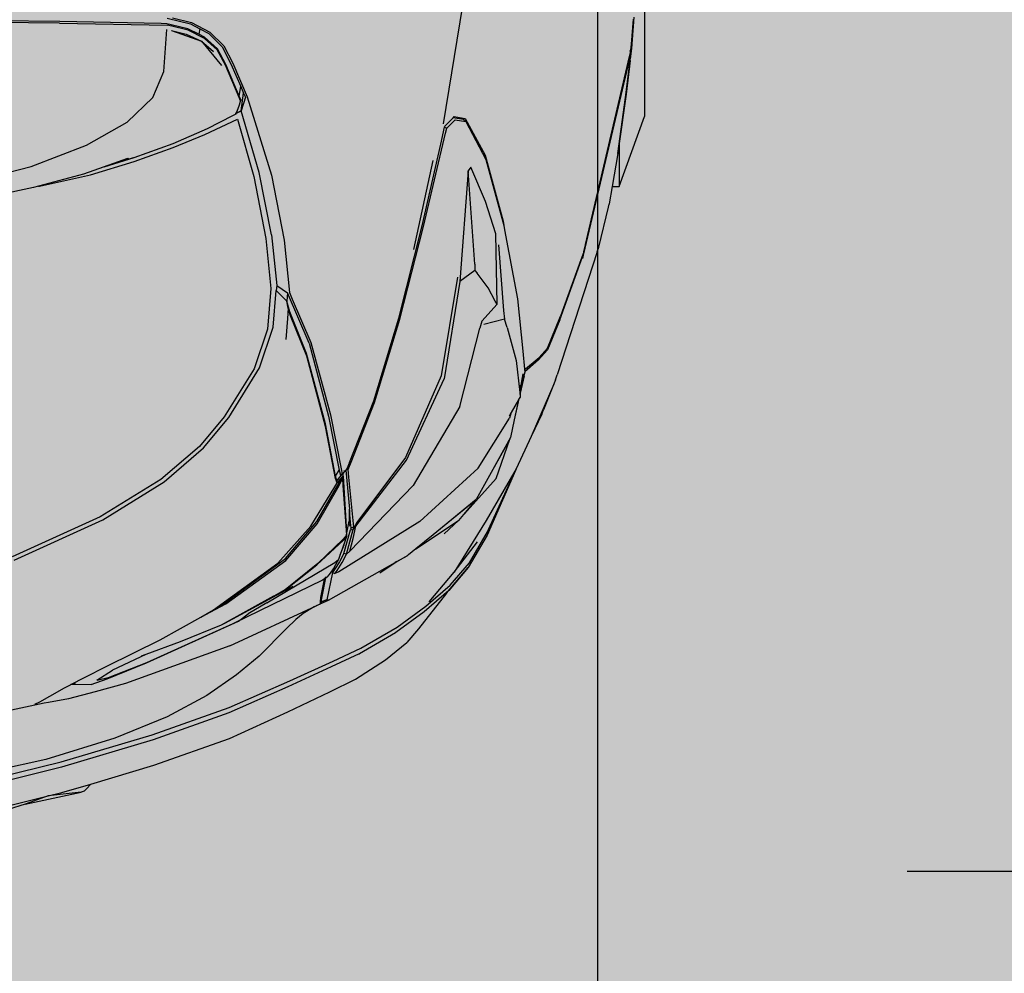
# Model space of a CAD drawing. Units: inches. Extents: x 1884 to 2398, y 474 to 1488.
# Tile 8 of 39: x 2247 to 2275, y 577 to 604. Entities that reach past the tile are written whole.
import ezdxf

# ---------------------------------------------------------------- set-up
doc = ezdxf.new("R2010")
doc.units = ezdxf.units.IN
doc.header["$MEASUREMENT"] = 0
doc.layers.get('0').update_dxf_attribs({"color": 250})
doc.layers.add('A-ANNO-DIMS', color=2, linetype='Continuous', lineweight=18)
doc.layers.add('C-VEHI', color=8, linetype='Continuous', lineweight=18)
doc.layers.add('Edges', color=250, linetype='Continuous')
doc.layers.add('L-PVMT-PATT', color=9, linetype='Continuous', lineweight=13, true_color=0xc7c8ca)
doc.styles.get("Standard").update_dxf_attribs({"font": 'arial.ttf'})
doc.dimstyles.get("Standard").update_dxf_attribs({"dimtxt": 7, "dimasz": 0.18, "dimexe": 0.18, "dimexo": 0.0625, "dimgap": 0.09, "dimtad": 0, "dimtih": 1, "dimtoh": 1, "dimzin": 0, "dimdsep": 46, "dimlunit": 3, "dimtxsty": 'Standard', "dimcen": 0.09, "dimadec": 0, "dimazin": 0, "dimtfac": 1, "dimtofl": 0, "dimtmove": 0, "dimatfit": 3, "dimfxl": 1, "dimtolj": 1, "dimtzin": 0, "dimarcsym": 0})

# ---------------------------------------------------------------- blocks, each defined once
blk = doc.blocks.new('Nissan Qashqai pl')
at = {"layer": 'Edges'}
for p, q in [((10.95774, 12.81008), (11.12826, 12.81008)), ((11.17826, 12.79208), (11.12826, 12.81008)), ((11.05762, 12.80257), (11.07977, 12.80077)), ((11.07681, 12.80079), (11.05899, 12.80228)), ((11.08106, 12.80045), (11.07681, 12.80079)), ((11.07977, 12.80077), (11.08723, 12.79991)), ((11.08273, 12.80006), (11.08106, 12.80045)), ((11.08273, 12.80006), (11.08133, 12.79984)), ((11.08365, 12.80022), (11.08273, 12.80006)), ((11.08562, 12.7994), (11.08273, 12.80006)), ((11.08723, 12.79991), (11.08365, 12.80022)), ((11.08365, 12.80022), (11.08821, 12.79916)), ((11.21955, 12.76812), (11.08562, 12.7994)), ((11.08834, 12.79978), (11.08723, 12.79991)), ((11.08821, 12.79916), (11.2222, 12.7676)), ((11.08834, 12.79978), (11.11234, 12.797)), ((11.11474, 12.79654), (11.08834, 12.79978)), ((11.11234, 12.797), (11.14751, 12.79208)), ((11.15472, 12.79099), (11.11474, 12.79654)), ((11.14751, 12.79208), (11.15248, 12.79138)), ((11.14751, 12.79208), (11.17826, 12.79208)), ((11.15248, 12.79138), (11.15472, 12.79099)), ((11.15472, 12.79099), (11.17826, 12.78701)), ((11.17826, 12.78701), (11.17826, 12.79208)), ((11.17826, 12.78701), (11.19065, 12.78493)), ((11.19065, 12.78493), (11.19089, 12.78487)), ((11.19297, 12.78452), (11.19089, 12.78487)), ((11.22148, 12.77754), (11.19297, 12.78452)), ((11.22475, 12.77644), (11.22148, 12.77754)), ((11.22475, 12.77644), (11.31244, 12.74788)), ((11.2247, 12.76695), (11.21633, 12.76893)), ((11.21998, 12.76802), (11.21955, 12.76812)), ((11.2247, 12.76695), (11.21998, 12.76802)), ((11.2222, 12.7676), (11.22715, 12.76645)), ((11.22532, 12.76679), (11.2247, 12.76695)), ((11.23038, 12.76493), (11.22532, 12.76679)), ((11.22532, 12.76679), (11.22706, 12.76639)), ((11.22715, 12.76645), (11.22962, 12.76579)), ((11.22715, 12.76645), (11.22772, 12.76624)), ((11.22772, 12.76624), (11.22962, 12.76579)), ((11.2732, 12.74964), (11.22772, 12.76624)), ((11.27044, 12.75036), (11.23038, 12.76493)), ((11.27015, 12.75067), (11.27044, 12.75036)), ((11.27037, 12.7506), (11.27066, 12.75028)), ((11.27066, 12.75028), (11.27044, 12.75036)), ((11.27187, 12.74984), (11.27066, 12.75028)), ((11.29339, 12.74103), (11.27187, 12.74984)), ((11.2732, 12.74964), (11.29459, 12.74089)), ((11.31612, 12.74669), (11.31244, 12.74788)), ((11.31612, 12.74669), (11.33757, 12.73813)), ((11.31923, 12.74536), (11.35656, 12.7294)), ((11.30003, 12.735), (11.29339, 12.74103)), ((11.29459, 12.74089), (11.30178, 12.73455)), ((11.30813, 12.72533), (11.30003, 12.735)), ((11.30178, 12.73455), (11.31027, 12.72493)), ((11.34052, 12.73691), (11.33757, 12.73813)), ((11.34052, 12.73691), (11.35656, 12.7294)), ((11.35656, 12.7294), (11.37962, 12.71869)), ((11.25827, 12.71956), (11.29558, 12.72339)), ((11.29558, 12.72339), (11.30849, 12.72466)), ((11.30218, 12.71856), (11.32517, 12.7213)), ((11.30863, 12.72468), (11.30813, 12.72533)), ((11.30813, 12.72533), (11.30866, 12.72468)), ((11.30849, 12.72466), (11.30863, 12.72468)), ((11.30863, 12.72468), (11.30866, 12.72468)), ((11.30866, 12.72468), (11.31033, 12.72486)), ((11.31027, 12.72493), (11.31033, 12.72486)), ((11.31033, 12.72486), (11.31061, 12.72489)), ((11.31061, 12.72489), (11.314, 12.72377)), ((11.31704, 12.72274), (11.31186, 12.72358)), ((11.31323, 12.7243), (11.32564, 12.72151)), ((11.314, 12.72377), (11.31704, 12.72274)), ((11.314, 12.72377), (11.32423, 12.72158)), ((11.32423, 12.72158), (11.31704, 12.72274)), ((11.31982, 12.72106), (11.32517, 12.7213)), ((11.32423, 12.72158), (11.32564, 12.72151)), ((11.32517, 12.7213), (11.32831, 12.72138)), ((11.32564, 12.72151), (11.32831, 12.72138)), ((11.32831, 12.72138), (11.32971, 12.7206)), ((11.32971, 12.7206), (11.34455, 12.71727)), ((11.32971, 12.7206), (11.33021, 12.72032)), ((11.33021, 12.72032), (11.34455, 12.71727)), ((11.33021, 12.72032), (11.33938, 12.71519)), ((11.20915, 12.71035), (11.25827, 12.71956)), ((11.27871, 12.71232), (11.30218, 12.71856)), ((11.33938, 12.71519), (11.34336, 12.71384)), ((11.33938, 12.71519), (11.34202, 12.71371)), ((11.37896, 12.69151), (11.34336, 12.71384)), ((11.34455, 12.71727), (11.3571, 12.7146)), ((11.35832, 12.71418), (11.3571, 12.7146)), ((11.3571, 12.7146), (11.38206, 12.70076)), ((11.35832, 12.71418), (11.38206, 12.70076)), ((11.3864, 12.70438), (11.35832, 12.71418)), ((11.37962, 12.71869), (11.41637, 12.69736)), ((11.37962, 12.71869), (11.38067, 12.71822)), ((11.38067, 12.71822), (11.42671, 12.69787)), ((11.42283, 12.69891), (11.38067, 12.71822)), ((11.15597, 12.69657), (11.20296, 12.70929)), ((11.15893, 12.69712), (11.20616, 12.70979)), ((11.20296, 12.70929), (11.20915, 12.71035)), ((11.20616, 12.70979), (11.20915, 12.71035)), ((11.21991, 12.70596), (11.26663, 12.70967)), ((11.26663, 12.70967), (11.27289, 12.71037)), ((11.27871, 12.71232), (11.27289, 12.71037)), ((11.27289, 12.71037), (11.27664, 12.69571)), ((11.2121, 12.70426), (11.18896, 12.69682)), ((11.26224, 12.70515), (11.2121, 12.70426)), ((11.26005, 12.70367), (11.25046, 12.69866)), ((11.26224, 12.70515), (11.26005, 12.70367)), ((11.27429, 12.69423), (11.26224, 12.70515)), ((11.38206, 12.70076), (11.40144, 12.69002)), ((11.41633, 12.67755), (11.3864, 12.70438)), ((11.12977, 12.68233), (11.15597, 12.69657)), ((11.13652, 12.68511), (11.15893, 12.69712)), ((11.18896, 12.69682), (11.16444, 12.68624)), ((11.25046, 12.69866), (11.2401, 12.69079)), ((11.27429, 12.69423), (11.27913, 12.69269)), ((11.33497, 12.6786), (11.27913, 12.69269)), ((11.41637, 12.69736), (11.45306, 12.67442)), ((11.42433, 12.69824), (11.42283, 12.69891)), ((11.44642, 12.68534), (11.42433, 12.69824)), ((11.42671, 12.69787), (11.44983, 12.68439)), ((11.13192, 12.68272), (11.13652, 12.68511)), ((11.16444, 12.68624), (11.16717, 12.6844)), ((11.23369, 12.68918), (11.16717, 12.6844)), ((11.23369, 12.68918), (11.23823, 12.68922)), ((11.23823, 12.68922), (11.2401, 12.69079)), ((11.23823, 12.68922), (11.24587, 12.67853)), ((11.37896, 12.69151), (11.41698, 12.64991)), ((11.40144, 12.69002), (11.40216, 12.6894)), ((11.40144, 12.69002), (11.42647, 12.65943)), ((11.40216, 12.6894), (11.41633, 12.67755)), ((11.40216, 12.6894), (11.42647, 12.65943)), ((11.45306, 12.67442), (11.43143, 12.69107)), ((11.46237, 12.67168), (11.44642, 12.68534)), ((11.13359, 12.66697), (11.04919, 12.68069)), ((11.12846, 12.67445), (11.12977, 12.68233)), ((11.13057, 12.68117), (11.12929, 12.67364)), ((11.13192, 12.68272), (11.13057, 12.68117)), ((11.13062, 12.67517), (11.13192, 12.68272)), ((11.16717, 12.6844), (11.24587, 12.67853)), ((11.24587, 12.67853), (11.31527, 12.66725)), ((11.33497, 12.6786), (11.3915, 12.64531)), ((11.44983, 12.68439), (11.46617, 12.67058)), ((11.46806, 12.66911), (11.44983, 12.68439)), ((11.12929, 12.67364), (11.12846, 12.67445)), ((11.13526, 12.66774), (11.12929, 12.67364)), ((11.1347, 12.67103), (11.13062, 12.67517)), ((11.24278, 12.67687), (11.31316, 12.66524)), ((11.43658, 12.64708), (11.41633, 12.67755)), ((11.41633, 12.67755), (11.42587, 12.66738)), ((11.4742, 12.65665), (11.45306, 12.67442)), ((11.47745, 12.65433), (11.46237, 12.67168)), ((11.13658, 12.66914), (11.1347, 12.67103)), ((11.13585, 12.66762), (11.13526, 12.66774)), ((11.13585, 12.66762), (11.13658, 12.66914)), ((11.14803, 12.66503), (11.13585, 12.66762)), ((11.14012, 12.66823), (11.13658, 12.66914)), ((11.20665, 12.65271), (11.14012, 12.66823)), ((11.20627, 12.65154), (11.14803, 12.66503)), ((11.31316, 12.66524), (11.3715, 12.63982)), ((11.37334, 12.64041), (11.31527, 12.66725)), ((11.46617, 12.67058), (11.48154, 12.65314)), ((11.46806, 12.66911), (11.49363, 12.64915)), ((11.22316, 12.64578), (11.1598, 12.65943)), ((11.42647, 12.65943), (11.43658, 12.64708)), ((11.27199, 12.63493), (11.20627, 12.65154)), ((11.27276, 12.63574), (11.20665, 12.65271)), ((11.49236, 12.63389), (11.47745, 12.65433)), ((11.48154, 12.65314), (11.49628, 12.63278)), ((11.3915, 12.64531), (11.4381, 12.60019)), ((11.41698, 12.64991), (11.45295, 12.59221)), ((11.43658, 12.64708), (11.44081, 12.64192)), ((11.49363, 12.64915), (11.50327, 12.64075)), ((11.3715, 12.63982), (11.41772, 12.60521)), ((11.42033, 12.60441), (11.37334, 12.64041)), ((11.44081, 12.64192), (11.4411, 12.64139)), ((11.4411, 12.64139), (11.44114, 12.64135)), ((11.44141, 12.64086), (11.44114, 12.64135)), ((11.44141, 12.64086), (11.44695, 12.63147)), ((11.44555, 12.63358), (11.44141, 12.64086)), ((11.51576, 12.62558), (11.50327, 12.64075)), ((11.33108, 12.61717), (11.27199, 12.63493)), ((11.33228, 12.61779), (11.27276, 12.63574)), ((11.44695, 12.63147), (11.44555, 12.63358)), ((11.44555, 12.63358), (11.4462, 12.63244)), ((11.44695, 12.63147), (11.4462, 12.63244)), ((11.47322, 12.58496), (11.4462, 12.63244)), ((11.44695, 12.63147), (11.44697, 12.63144)), ((11.45359, 12.62148), (11.44697, 12.63144)), ((11.50736, 12.608), (11.49236, 12.63389)), ((11.49639, 12.63259), (11.49628, 12.63278)), ((11.49639, 12.63259), (11.51127, 12.60694)), ((11.52949, 12.60412), (11.51576, 12.62558)), ((11.37505, 12.59987), (11.33108, 12.61717)), ((11.37475, 12.60107), (11.33228, 12.61779)), ((11.51652, 12.58815), (11.50736, 12.608)), ((11.38, 12.59884), (11.37475, 12.60107)), ((11.42115, 12.60299), (11.38533, 12.59929)), ((11.42154, 12.60103), (11.41765, 12.60067)), ((11.41772, 12.60521), (11.41931, 12.60418)), ((11.41915, 12.60447), (11.4194, 12.6042)), ((11.4194, 12.6042), (11.41931, 12.60418)), ((11.41931, 12.60418), (11.4196, 12.60399)), ((11.41958, 12.60424), (11.4194, 12.6042)), ((11.4194, 12.6042), (11.4196, 12.60399)), ((11.4196, 12.60399), (11.42014, 12.60365)), ((11.41984, 12.60411), (11.42014, 12.60365)), ((11.42014, 12.60365), (11.42115, 12.60299)), ((11.42915, 12.60239), (11.42033, 12.60441)), ((11.42287, 12.60252), (11.42033, 12.60441)), ((11.42115, 12.60299), (11.42154, 12.60103)), ((11.42178, 12.60282), (11.42115, 12.60299)), ((11.42154, 12.60103), (11.4219, 12.60093)), ((11.42216, 12.6029), (11.42178, 12.60282)), ((11.42287, 12.60252), (11.42178, 12.60282)), ((11.4219, 12.60093), (11.42218, 12.6005)), ((11.4219, 12.60093), (11.42243, 12.60078)), ((11.43154, 12.6002), (11.42287, 12.60252)), ((11.42296, 12.60064), (11.42287, 12.60252)), ((11.4381, 12.60019), (11.42915, 12.60239)), ((11.51135, 12.60676), (11.51127, 12.60694)), ((11.51135, 12.60676), (11.52058, 12.58692)), ((11.53843, 12.58586), (11.52949, 12.60412)), ((11.37505, 12.59987), (11.37621, 12.59987)), ((11.37522, 12.5998), (11.37505, 12.59987)), ((11.3763, 12.5998), (11.37522, 12.5998)), ((11.3764, 12.59934), (11.37522, 12.5998)), ((11.37922, 12.59823), (11.3764, 12.59934)), ((11.37922, 12.59823), (11.37931, 12.59792)), ((11.37922, 12.59823), (11.38041, 12.59725)), ((11.37955, 12.59389), (11.38338, 12.59468)), ((11.38533, 12.59929), (11.38, 12.59884)), ((11.38041, 12.59725), (11.40818, 12.5998)), ((11.38275, 12.5953), (11.38041, 12.59725)), ((11.38113, 12.59582), (11.38084, 12.59606)), ((11.38338, 12.59468), (11.38275, 12.5953)), ((11.38461, 12.59531), (11.38295, 12.59519)), ((11.38295, 12.59519), (11.38491, 12.59506)), ((11.38801, 12.59095), (11.38295, 12.59519)), ((11.38338, 12.59468), (11.38408, 12.59335)), ((11.38465, 12.59529), (11.38461, 12.59531)), ((11.38465, 12.59529), (11.42481, 12.59763)), ((11.38507, 12.59505), (11.38465, 12.59529)), ((11.38465, 12.59529), (11.38491, 12.59506)), ((11.38491, 12.59506), (11.38507, 12.59505)), ((11.38823, 12.59226), (11.38491, 12.59506)), ((11.38507, 12.59505), (11.3867, 12.59494)), ((11.41708, 12.57658), (11.38507, 12.59505)), ((11.3867, 12.59494), (11.3915, 12.59511)), ((11.3914, 12.5926), (11.3867, 12.59494)), ((11.3915, 12.59511), (11.42659, 12.59766)), ((11.40898, 12.59987), (11.40818, 12.5998)), ((11.41644, 12.5998), (11.40818, 12.5998)), ((11.4152, 12.60045), (11.40898, 12.59987)), ((11.40898, 12.59987), (11.4163, 12.59987)), ((11.41735, 12.60064), (11.4152, 12.60045)), ((11.4163, 12.59987), (11.4152, 12.60045)), ((11.4163, 12.59987), (11.41856, 12.59987)), ((11.41644, 12.5998), (11.4163, 12.59987)), ((11.41814, 12.5998), (11.41644, 12.5998)), ((11.41686, 12.59958), (11.41644, 12.5998)), ((11.4252, 12.59796), (11.41686, 12.59958)), ((11.41765, 12.60067), (11.41735, 12.60064)), ((11.41798, 12.60055), (11.41735, 12.60064)), ((11.41798, 12.60055), (11.41765, 12.60067)), ((11.42045, 12.6002), (11.41798, 12.60055)), ((11.41944, 12.60003), (11.41798, 12.60055)), ((11.42243, 12.60078), (11.42261, 12.60058)), ((11.42243, 12.60078), (11.42296, 12.60064)), ((11.43996, 12.59594), (11.42296, 12.60064)), ((11.42481, 12.59763), (11.42659, 12.59766)), ((11.42659, 12.59766), (11.4252, 12.59796)), ((11.42659, 12.59766), (11.42684, 12.59767)), ((11.42684, 12.59767), (11.42784, 12.5977)), ((11.42684, 12.59767), (11.42958, 12.59536)), ((11.43028, 12.59564), (11.42784, 12.5977)), ((11.42784, 12.5977), (11.42996, 12.59695)), ((11.42958, 12.59536), (11.44691, 12.57732)), ((11.43368, 12.59616), (11.42996, 12.59695)), ((11.42996, 12.59695), (11.43609, 12.59479)), ((11.44788, 12.57656), (11.43028, 12.59564)), ((11.44027, 12.59779), (11.43154, 12.6002)), ((11.4397, 12.59367), (11.43368, 12.59616)), ((11.43609, 12.59479), (11.44061, 12.59321)), ((11.4381, 12.60019), (11.44027, 12.59779)), ((11.44027, 12.59779), (11.43996, 12.59594)), ((11.43996, 12.59594), (11.44573, 12.59285)), ((11.44624, 12.59468), (11.44027, 12.59779)), ((11.45199, 12.59099), (11.44624, 12.59468)), ((11.3411, 12.58627), (11.37955, 12.59389)), ((11.34188, 12.585), (11.38043, 12.59263)), ((11.3847, 12.58985), (11.34742, 12.58274)), ((11.38634, 12.58979), (11.34932, 12.58277)), ((11.38043, 12.59263), (11.38408, 12.59335)), ((11.3847, 12.58985), (11.38043, 12.59263)), ((11.3847, 12.58985), (11.38475, 12.58986)), ((11.38801, 12.59095), (11.38475, 12.58986)), ((11.38953, 12.59117), (11.38634, 12.58979)), ((11.38862, 12.59194), (11.3872, 12.59275)), ((11.38823, 12.59226), (11.38862, 12.59194)), ((11.38862, 12.59194), (11.38953, 12.59117)), ((11.38916, 12.59162), (11.38862, 12.59194)), ((11.39234, 12.58945), (11.38953, 12.59117)), ((11.41866, 12.57682), (11.3914, 12.5926)), ((11.42028, 12.57243), (11.39234, 12.58945)), ((11.44061, 12.59321), (11.4397, 12.59367)), ((11.44061, 12.59321), (11.44418, 12.59196)), ((11.44418, 12.59196), (11.44968, 12.58897)), ((11.4462, 12.58934), (11.44418, 12.59196)), ((11.44573, 12.59285), (11.45121, 12.58927)), ((11.47499, 12.54092), (11.4462, 12.58934)), ((11.44968, 12.58897), (11.44984, 12.58887)), ((11.45351, 12.58765), (11.44984, 12.58887)), ((11.44984, 12.58887), (11.45491, 12.58548)), ((11.45121, 12.58927), (11.45351, 12.58765)), ((11.45386, 12.58968), (11.45199, 12.59099)), ((11.45295, 12.59221), (11.45421, 12.58943)), ((11.45351, 12.58765), (11.45316, 12.58821)), ((11.45351, 12.58765), (11.45421, 12.58943)), ((11.45351, 12.58765), (11.47278, 12.58377)), ((11.45421, 12.58943), (11.45386, 12.58968)), ((11.53062, 12.55726), (11.51652, 12.58815)), ((11.52058, 12.58692), (11.53487, 12.5559)), ((11.28951, 12.57239), (11.3411, 12.58627)), ((11.29, 12.57107), (11.34188, 12.585)), ((11.34739, 12.58273), (11.29721, 12.56923)), ((11.34932, 12.58277), (11.29928, 12.56948)), ((11.34739, 12.58273), (11.34742, 12.58274)), ((11.45491, 12.58548), (11.45678, 12.58362)), ((11.4564, 12.5833), (11.45669, 12.58328)), ((11.45688, 12.58305), (11.45652, 12.58312)), ((11.45678, 12.58362), (11.45714, 12.58326)), ((11.45714, 12.58326), (11.45732, 12.58296)), ((11.45734, 12.58226), (11.45729, 12.58229)), ((11.45732, 12.58296), (11.45781, 12.58216)), ((11.47041, 12.58031), (11.45732, 12.58296)), ((11.45734, 12.58226), (11.45736, 12.58221)), ((11.45755, 12.58222), (11.45736, 12.58221)), ((11.45781, 12.58216), (11.45883, 12.58071)), ((11.46047, 12.58162), (11.45781, 12.58216)), ((11.45883, 12.58071), (11.48954, 12.5178)), ((11.47129, 12.57943), (11.46047, 12.58162)), ((11.47423, 12.5797), (11.47041, 12.58031)), ((11.47322, 12.58496), (11.47278, 12.58377)), ((11.47278, 12.58377), (11.47423, 12.5797)), ((11.47278, 12.58377), (11.47463, 12.57959)), ((11.47585, 12.57907), (11.47322, 12.58496)), ((11.55274, 12.55595), (11.53843, 12.58586)), ((11.44331, 12.55428), (11.41708, 12.57658)), ((11.44474, 12.55451), (11.41866, 12.57682)), ((11.44691, 12.57732), (11.46587, 12.55394)), ((11.46538, 12.55485), (11.44788, 12.57656)), ((11.47442, 12.57918), (11.47129, 12.57943)), ((11.47423, 12.5797), (11.47442, 12.57918)), ((11.47445, 12.57967), (11.47423, 12.5797)), ((11.47446, 12.57918), (11.47442, 12.57918)), ((11.47446, 12.57918), (11.47445, 12.57967)), ((11.47445, 12.57967), (11.47463, 12.57959)), ((11.47482, 12.57915), (11.47446, 12.57918)), ((11.47463, 12.57959), (11.47482, 12.57915)), ((11.47463, 12.57959), (11.47585, 12.57907)), ((11.47585, 12.57907), (11.47482, 12.57915)), ((11.47585, 12.57907), (11.47588, 12.57899)), ((11.47588, 12.57899), (11.47783, 12.57463)), ((11.47588, 12.57899), (11.47707, 12.57604)), ((11.50574, 12.51451), (11.47707, 12.57604)), ((11.47783, 12.57463), (11.48256, 12.56692)), ((11.29, 12.57107), (11.2541, 12.55571)), ((11.25857, 12.55913), (11.28951, 12.57239)), ((11.29721, 12.56923), (11.2677, 12.55747)), ((11.29928, 12.56948), (11.27055, 12.55794)), ((11.44669, 12.5488), (11.42028, 12.57243)), ((11.48256, 12.56692), (11.48692, 12.56154)), ((11.25377, 12.5571), (11.25857, 12.55913)), ((11.46332, 12.55943), (11.48966, 12.51079)), ((11.48692, 12.56154), (11.49329, 12.55504)), ((11.17021, 12.54438), (11.21656, 12.55336)), ((11.21656, 12.55336), (11.25377, 12.5571)), ((11.24875, 12.54799), (11.2541, 12.55571)), ((11.25993, 12.55525), (11.25238, 12.54768)), ((11.2541, 12.55571), (11.25993, 12.55525)), ((11.2677, 12.55747), (11.25993, 12.55525)), ((11.26503, 12.55627), (11.25993, 12.55525)), ((11.27055, 12.55794), (11.26503, 12.55627)), ((11.26503, 12.55627), (11.27242, 12.55569)), ((11.27242, 12.55569), (11.28736, 12.55442)), ((11.47454, 12.51164), (11.44331, 12.55428)), ((11.4758, 12.51184), (11.44474, 12.55451)), ((11.46538, 12.55485), (11.46587, 12.55394)), ((11.46587, 12.55394), (11.46737, 12.55123)), ((11.51313, 12.53562), (11.49329, 12.55504)), ((11.54963, 12.51414), (11.53062, 12.55726)), ((11.53487, 12.5559), (11.5535, 12.51389)), ((11.57164, 12.51447), (11.55274, 12.55595)), ((11.21271, 12.54434), (11.24875, 12.54799)), ((11.24875, 12.54799), (11.25238, 12.54768)), ((11.27848, 12.54551), (11.25238, 12.54768)), ((11.30757, 12.53583), (11.27848, 12.54551)), ((11.48013, 12.50304), (11.44669, 12.5488)), ((11.46746, 12.55104), (11.46737, 12.55123)), ((11.46746, 12.55104), (11.47026, 12.54595)), ((11.47026, 12.54595), (11.47038, 12.54575)), ((11.47038, 12.54575), (11.49086, 12.50849)), ((11.47038, 12.54575), (11.48966, 12.51079)), ((11.11439, 12.52705), (11.17021, 12.54438)), ((11.21271, 12.54434), (11.16835, 12.53543)), ((11.17121, 12.53172), (11.21523, 12.54036)), ((11.21523, 12.54036), (11.2509, 12.54386)), ((11.2509, 12.54386), (11.28005, 12.5414)), ((11.28005, 12.5414), (11.3082, 12.53202)), ((11.47499, 12.54092), (11.48281, 12.52763)), ((11.16835, 12.53543), (11.1244, 12.5227)), ((11.13017, 12.52), (11.17121, 12.53172)), ((11.34283, 12.5139), (11.30757, 12.53583)), ((11.3082, 12.53202), (11.34251, 12.51056)), ((11.51313, 12.53562), (11.52646, 12.51943)), ((11.09022, 12.51663), (11.11439, 12.52705)), ((11.10704, 12.52235), (11.11164, 12.52434)), ((11.11164, 12.52434), (11.11467, 12.52565)), ((11.1244, 12.5227), (11.11164, 12.52434)), ((11.11467, 12.52565), (11.1244, 12.5227)), ((11.48801, 12.52079), (11.48281, 12.52763)), ((11.09081, 12.51534), (11.10704, 12.52235)), ((11.1138, 12.52126), (11.09121, 12.51168)), ((11.11486, 12.52116), (11.09174, 12.51145)), ((11.1138, 12.52126), (11.10704, 12.52235)), ((11.11393, 12.52132), (11.1138, 12.52126)), ((11.1164, 12.52245), (11.11393, 12.52132)), ((11.1172, 12.5222), (11.11486, 12.52116)), ((11.1164, 12.52245), (11.11744, 12.52227)), ((11.11725, 12.52219), (11.1172, 12.5222)), ((11.11744, 12.52227), (11.11725, 12.52219)), ((11.11997, 12.52149), (11.11744, 12.52227)), ((11.12459, 12.51987), (11.11997, 12.52149)), ((11.12591, 12.5194), (11.1244, 12.5227)), ((11.1244, 12.5227), (11.12604, 12.51935)), ((11.12591, 12.5194), (11.12459, 12.51987)), ((11.12595, 12.51931), (11.12466, 12.51974)), ((11.12595, 12.51931), (11.12478, 12.51949)), ((11.1251, 12.51886), (11.12595, 12.51931)), ((11.12595, 12.51931), (11.12591, 12.5194)), ((11.12604, 12.51935), (11.12591, 12.5194)), ((11.12626, 12.51863), (11.12595, 12.51931)), ((11.12607, 12.51928), (11.12595, 12.51931)), ((11.12604, 12.51935), (11.12607, 12.51928)), ((11.12645, 12.51921), (11.12604, 12.51935)), ((11.12607, 12.51928), (11.12631, 12.51879)), ((11.12645, 12.51921), (11.12607, 12.51928)), ((11.12767, 12.51667), (11.12645, 12.51921)), ((11.14123, 12.4969), (11.13017, 12.52)), ((11.51787, 12.45515), (11.48801, 12.52079)), ((11.48983, 12.51722), (11.48954, 12.5178)), ((11.48983, 12.51722), (11.49005, 12.51666)), ((11.52646, 12.51943), (11.54097, 12.49823)), ((11.06818, 12.50039), (11.07787, 12.51026)), ((11.07787, 12.51026), (11.09022, 12.51663)), ((11.07866, 12.50924), (11.09081, 12.51534)), ((11.09121, 12.51168), (11.08018, 12.50575)), ((11.09174, 12.51145), (11.0809, 12.50558)), ((11.13692, 12.49861), (11.12767, 12.51667)), ((11.34251, 12.51056), (11.3635, 12.49291)), ((11.36451, 12.49581), (11.34283, 12.5139)), ((11.47876, 12.50515), (11.47454, 12.51164)), ((11.48518, 12.49399), (11.4758, 12.51184)), ((11.48966, 12.51079), (11.49086, 12.50849)), ((11.49005, 12.51666), (11.51787, 12.45515)), ((11.50574, 12.51451), (11.53253, 12.44036)), ((11.56912, 12.45916), (11.54963, 12.51414)), ((11.5535, 12.51389), (11.57263, 12.45997)), ((11.59084, 12.46055), (11.57164, 12.51447)), ((11.06918, 12.49965), (11.07866, 12.50924)), ((11.08018, 12.50575), (11.07183, 12.49667)), ((11.0809, 12.50558), (11.0727, 12.49662)), ((11.07472, 12.49435), (11.092, 12.50868)), ((11.07472, 12.49435), (11.08206, 12.50291)), ((11.48013, 12.50304), (11.47876, 12.50515)), ((11.48518, 12.49399), (11.48013, 12.50304)), ((11.49086, 12.50849), (11.50277, 12.47921)), ((11.06139, 12.48725), (11.06818, 12.50039)), ((11.06584, 12.49324), (11.06918, 12.49965)), ((11.0727, 12.49662), (11.06692, 12.48495)), ((11.07183, 12.49667), (11.06978, 12.49253)), ((11.14751, 12.47415), (11.13692, 12.49861)), ((11.15051, 12.47418), (11.14123, 12.4969)), ((11.38877, 12.46778), (11.36451, 12.49581)), ((11.54097, 12.49823), (11.55624, 12.47006)), ((11.06236, 12.48656), (11.06584, 12.49324)), ((11.06584, 12.49324), (11.06978, 12.49253)), ((11.06978, 12.49253), (11.06594, 12.48477)), ((11.0671, 12.47307), (11.07472, 12.49435)), ((11.06961, 12.4836), (11.07472, 12.49435)), ((11.3635, 12.49291), (11.38718, 12.46538)), ((11.50131, 12.46508), (11.48518, 12.49399)), ((11.05807, 12.47379), (11.06139, 12.48725)), ((11.05822, 12.46998), (11.06236, 12.48656)), ((11.06594, 12.48477), (11.06303, 12.47281)), ((11.06692, 12.48495), (11.06408, 12.47331)), ((11.0671, 12.47307), (11.06961, 12.4836)), ((11.50277, 12.47921), (11.5118, 12.45478)), ((11.06182, 12.39327), (11.06324, 12.47002)), ((11.06222, 12.46967), (11.06214, 12.46571)), ((11.06303, 12.47281), (11.06222, 12.46967)), ((11.06408, 12.47331), (11.06324, 12.47002)), ((11.09618, 12.46753), (11.06624, 12.46981)), ((11.15766, 12.44645), (11.14751, 12.47415)), ((11.16047, 12.4465), (11.15051, 12.47418)), ((11.41588, 12.42419), (11.38877, 12.46778)), ((11.55624, 12.47006), (11.57152, 12.43265)), ((11.06214, 12.46571), (11.06074, 12.39335)), ((11.11477, 12.45982), (11.09618, 12.46753)), ((11.38718, 12.46538), (11.41383, 12.4223)), ((11.5202, 12.42705), (11.50131, 12.46508)), ((11.1323, 12.44148), (11.11477, 12.45982)), ((11.5118, 12.45478), (11.52299, 12.43109)), ((11.5118, 12.45478), (11.51304, 12.45142)), ((11.52922, 12.42717), (11.51787, 12.45515)), ((11.51787, 12.45515), (11.52855, 12.42791)), ((11.58843, 12.39431), (11.56912, 12.45916)), ((11.57263, 12.45997), (11.59225, 12.39471)), ((11.60419, 12.41556), (11.59084, 12.46055)), ((11.14869, 12.41255), (11.1323, 12.44148)), ((11.16426, 12.42498), (11.15764, 12.44588)), ((11.16426, 12.42498), (11.15766, 12.44645)), ((11.1582, 12.44157), (11.1668, 12.41765)), ((11.15826, 12.4423), (11.16426, 12.42498)), ((11.1699, 12.41527), (11.16047, 12.4465)), ((11.53253, 12.44036), (11.53855, 12.41873)), ((11.57152, 12.43265), (11.58664, 12.38348)), ((11.52833, 12.41095), (11.5202, 12.42705)), ((11.53009, 12.41977), (11.52299, 12.43109)), ((11.52855, 12.42791), (11.53022, 12.42092)), ((11.53313, 12.41568), (11.52922, 12.42717)), ((11.16426, 12.42498), (11.1668, 12.41765)), ((11.41383, 12.4223), (11.44218, 12.3594)), ((11.44453, 12.36082), (11.41588, 12.42419)), ((11.53022, 12.42092), (11.53009, 12.41977)), ((11.53855, 12.41873), (11.54336, 12.39967)), ((11.16395, 12.37304), (11.14869, 12.41255)), ((11.1668, 12.41765), (11.1694, 12.41042)), ((11.17797, 12.37897), (11.1699, 12.41527)), ((11.53313, 12.41568), (11.53354, 12.40102)), ((11.60419, 12.41556), (11.60772, 12.41254)), ((11.61028, 12.39501), (11.60419, 12.41556)), ((11.60772, 12.41254), (11.60938, 12.41069)), ((11.1694, 12.41042), (11.17808, 12.37824)), ((11.53335, 12.40136), (11.52833, 12.41095)), ((11.53261, 12.40451), (11.5333, 12.40191)), ((11.60938, 12.41069), (11.61008, 12.40855)), ((11.61008, 12.40855), (11.61272, 12.38521)), ((11.61848, 12.36888), (11.61008, 12.40855)), ((11.5333, 12.40191), (11.53335, 12.40136)), ((11.53354, 12.40102), (11.53335, 12.40136)), ((11.53572, 12.39685), (11.53354, 12.40102)), ((11.54336, 12.39967), (11.54611, 12.38542)), ((11.06074, 12.39335), (11.05947, 12.28422)), ((11.06182, 12.39327), (11.06059, 12.28408)), ((11.54162, 12.38633), (11.53572, 12.39685)), ((11.60765, 12.31656), (11.58843, 12.39431)), ((11.59225, 12.39471), (11.61178, 12.31654)), ((11.61272, 12.38521), (11.61028, 12.39501)), ((11.54554, 12.37932), (11.54162, 12.38633)), ((11.54611, 12.38542), (11.54666, 12.38219)), ((11.58664, 12.38348), (11.6016, 12.31655)), ((11.61272, 12.38521), (11.61742, 12.37218)), ((11.62966, 12.31657), (11.61272, 12.38521)), ((11.17808, 12.37824), (11.17797, 12.37897)), ((11.17808, 12.37824), (11.17906, 12.37461)), ((11.54721, 12.37575), (11.54554, 12.37932)), ((11.54666, 12.38219), (11.55707, 12.33312)), ((11.17758, 12.32109), (11.16395, 12.37304)), ((11.17906, 12.37461), (11.18773, 12.33305)), ((11.61742, 12.37218), (11.61848, 12.36888)), ((11.61848, 12.36888), (11.62241, 12.35673))]:
    blk.add_line(p, q, dxfattribs=at)
blk = doc.blocks.new('car')
blk.add_blockref('Nissan Qashqai pl', (-9.74328, -11.91512))
blk = doc.blocks.new('carr')
blk.add_blockref('car', (0.51244, -0.00696))
blk = doc.blocks.new('*D23')
at = {"layer": 'A-ANNO-DIMS', "color": 0, "lineweight": -2, "transparency": 16777216}
for p, q in [((2272.304, 752.812), (2298.291, 752.812)), ((2298.111, 752.632), (2298.111, 670.29)), ((2298.111, 580.529), (2298.111, 662.871)), ((2272.304, 580.349), (2298.291, 580.349))]:
    blk.add_line(p, q, dxfattribs=at)
at = {"layer": 'A-ANNO-DIMS', "color": 0, "lineweight": 100, "transparency": 16777216}
for points in [[(2298.081, 752.632), (2298.141, 752.632), (2298.111, 752.812)], [(2298.081, 580.529), (2298.141, 580.529), (2298.111, 580.349)]]:
    blk.add_solid(points, dxfattribs=at)
at = {"layer": 'Defpoints', "color": 0, "lineweight": 100, "transparency": 16777216}
for p in [(2272.242, 752.812), (2272.242, 580.349), (2298.111, 580.349)]:
    blk.add_point(p, dxfattribs=at)
at = {"layer": 'A-ANNO-DIMS', "color": 0, "transparency": 16777216, "insert": (2298.111, 666.58), "char_height": 7, "attachment_point": 5}
blk.add_mtext('\\A1;CAR 14\'-4 1/2" TYP.', dxfattribs=at)
blk = doc.blocks.new('*D44')
at = {"layer": 'A-ANNO-DIMS', "color": 0, "lineweight": -2, "transparency": 16777216}
for p, q in [((2209.755, 1247.822), (2209.755, 484.005)), ((2230.029, 1247.822), (2230.029, 484.005)), ((2209.935, 484.185), (2229.849, 484.185)), ((2230.029, 484.185), (2230.209, 484.185))]:
    blk.add_line(p, q, dxfattribs=at)
at = {"layer": 'A-ANNO-DIMS', "color": 0, "lineweight": 100, "transparency": 16777216}
for points in [[(2209.935, 484.215), (2209.935, 484.155), (2209.755, 484.185)], [(2229.849, 484.215), (2229.849, 484.155), (2230.029, 484.185)]]:
    blk.add_solid(points, dxfattribs=at)
at = {"layer": 'Defpoints', "color": 0, "lineweight": 100, "transparency": 16777216}
for p in [(2209.755, 1247.885), (2230.029, 1247.885), (2230.029, 484.185)]:
    blk.add_point(p, dxfattribs=at)
at = {"layer": 'A-ANNO-DIMS', "color": 0, "transparency": 16777216, "insert": (2247.429, 484.185), "char_height": 7, "attachment_point": 5}
blk.add_mtext('\\A1;1\'-8 1/2"', dxfattribs=at)
blk = doc.blocks.new('*D45')
at = {"layer": 'A-ANNO-DIMS', "color": 0, "lineweight": -2, "transparency": 16777216}
for p, q in [((2242.617, 1322.822), (2242.617, 484.005)), ((2263.617, 1322.822), (2263.617, 484.005)), ((2242.797, 484.185), (2244.052, 484.185)), ((2263.437, 484.185), (2262.181, 484.185))]:
    blk.add_line(p, q, dxfattribs=at)
at = {"layer": 'A-ANNO-DIMS', "color": 0, "lineweight": 100, "transparency": 16777216}
for points in [[(2242.797, 484.215), (2242.797, 484.155), (2242.617, 484.185)], [(2263.437, 484.215), (2263.437, 484.155), (2263.617, 484.185)]]:
    blk.add_solid(points, dxfattribs=at)
at = {"layer": 'Defpoints', "color": 0, "lineweight": 100, "transparency": 16777216}
for p in [(2242.617, 1322.885), (2263.617, 1322.885), (2263.617, 484.185)]:
    blk.add_point(p, dxfattribs=at)
at = {"layer": 'A-ANNO-DIMS', "color": 0, "transparency": 16777216, "insert": (2253.117, 484.185), "char_height": 7, "attachment_point": 5}
blk.add_mtext('\\A1;1\'-9"', dxfattribs=at)

msp = doc.modelspace()

# ---------------------------------------------------------------- hatches: boundary and pattern name
at = {"layer": 'L-PVMT-PATT'}
h = msp.add_hatch(color=256, dxfattribs=at)
h.dxf.hatch_style = 1
h.paths.add_polyline_path([(2387.529, 769.966), (2351.529, 769.966), (2238.447, 769.966), (2238.447, 762.15), (2238.447, 754.445), (2126.529, 754.445), (2126.529, 676.183), (2134.868, 676.183), (2142.673, 676.183), (2142.673, 646.578), (2134.868, 646.578), (2126.529, 646.578), (2126.529, 640.17), (2387.529, 640.17)])
h.paths.add_polyline_path([(2387.529, 631.385), (2303.086, 631.385), (2303.086, 615.671), (2387.529, 615.671)])
h.paths.add_polyline_path([(2387.529, 640.17), (2126.529, 640.17), (2126.529, 631.385), (2387.529, 631.385)])
h.paths.add_polyline_path([(2393.529, 604.13), (2387.529, 604.13), (2387.529, 615.671), (2303.086, 615.671), (2303.086, 607.943), (2249.649, 607.943), (2126.529, 607.943), (2126.529, 533.885), (2393.529, 533.885)])
h.paths.add_polyline_path([(2257.825, 611.008), (2257.83, 611.337), (2257.915, 616.493), (2258.021, 621.805), (2258.146, 627.274), (2258.252, 631.385), (2126.529, 631.385), (2126.529, 611.008)])
h.paths.add_polyline_path([(2258.892, 611.285), (2258.888, 611.008), (2300.247, 611.008), (2300.247, 631.385), (2259.314, 631.385), (2259.206, 627.173), (2259.081, 621.72), (2258.976, 616.424)])

# ---------------------------------------------------------------- block references
at = {"layer": 'C-VEHI', "xscale": 39.37007874015748, "yscale": 39.37007874015748, "zscale": 39.37007874015748, "rotation": 270}
msp.add_blockref('carr', (2229.977, 676.232), dxfattribs=at)

# ---------------------------------------------------------------- dimensions: what is measured, and where the dimension line sits
at = {"layer": 'A-ANNO-DIMS'}
for base, p1, p2, picture, middle in [((2263.617, 484.185), (2242.617, 1322.885), (2263.617, 1322.885), '*D45', (2253.117, 484.185)), ((2230.029, 484.185), (2209.755, 1247.885), (2230.029, 1247.885), '*D44', (2247.429, 484.185))]:
    dim = msp.add_linear_dim(base=base, p1=p1, p2=p2, dimstyle='Standard', override={"dimdec": 1, "dimlfac": 1, "dimrnd": 0, "dimzin": 1, "dimdsep": 46, "dimlunit": 4, "dimfrac": 2}, dxfattribs=at)
    dim.commit()
    dim.dimension.update_dxf_attribs({"geometry": picture, "text_midpoint": middle})
dim = msp.add_linear_dim(base=(2298.111, 580.349), p1=(2272.242, 752.812), p2=(2272.242, 580.349), angle=270, text='CAR <> TYP.', dimstyle='Standard', override={"dimdec": 1, "dimlfac": 1, "dimrnd": 0, "dimzin": 1, "dimdsep": 46, "dimlunit": 4, "dimfrac": 2}, dxfattribs=at)
dim.commit()
dim.dimension.update_dxf_attribs({"geometry": '*D23', "text_midpoint": (2298.111, 666.58)})

doc.saveas('drawing.dxf')
